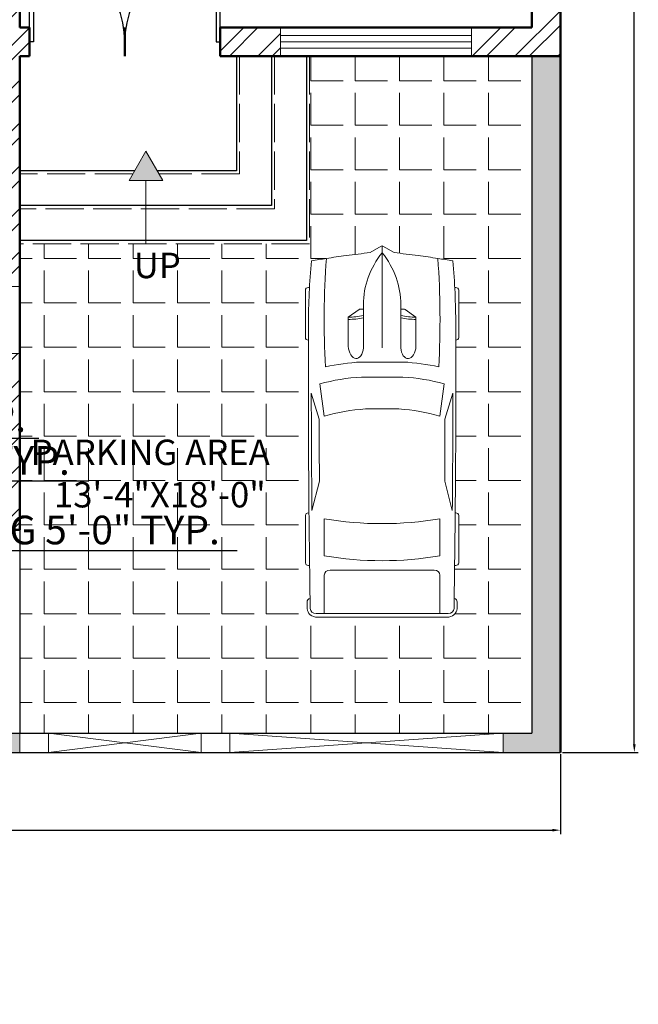
# Model space of a CAD drawing. Units: inches. Extents: x 764 to 1199, y 2696 to 3678.
# Tile 1 of 3: x 984 to 1179, y 2741 to 3051. Entities that reach past the tile are written whole.
import ezdxf

# ---------------------------------------------------------------- set-up
doc = ezdxf.new("R2010")
doc.units = ezdxf.units.IN
doc.linetypes.add('ACAD_ISO02W100', pattern=[15, 12, -3])
for name, color, linetype, lineweight in [('A-ANNO-DIMS', 2, 'Continuous', 18), ('A-ANNO-SYMB', 7, 'Continuous', 18), ('A-ANNO-TEXT', 7, 'Continuous', 18), ('A-AREA-IDEN', 7, 'Continuous', 18), ('A-DOOR', 4, 'Continuous', 25), ('A-FLOR-PATT', 9, 'Continuous', 13), ('A-FLOR-STRS', 7, 'Continuous', 25), ('A-GLAZ', 244, 'Continuous', 20), ('A-STRS-HIDN', 8, 'ACAD_ISO02W100', 13), ('A-WALL', 7, 'Continuous', 50), ('A-WALL-PATT', 252, 'Continuous', 13), ('C-PKG-VEHI', 8, 'Continuous', 18), ('L-GATE', 244, 'Continuous', 20), ('L-HRDS', 7, 'Continuous', 30)]:
    doc.layers.add(name, color=color, linetype=linetype, lineweight=lineweight)
doc.styles.get("Standard").update_dxf_attribs({"font": 'arial.ttf'})
doc.dimstyles.new('ISO-25', dxfattribs={"dimtxt": 9, "dimasz": 2.5, "dimexe": 1.25, "dimexo": 0.625, "dimtad": 1, "dimlunit": 3, "dimtxsty": 'Standard', "dimcen": 2.5, "dimadec": 0, "dimazin": 0, "dimtfac": 1, "dimtmove": 0, "dimatfit": 3, "dimfxl": 1, "dimarcsym": 0})
pattern_1 = [(45, (0, 0), (-6.735192090801866, 6.735192090801866), []), (45, (4.49013, 0), (-6.735192090801866, 6.735192090801866), [])]

# ---------------------------------------------------------------- blocks, each defined once
blk = doc.blocks.new('*U2')
for p, q in [((0, 0), (-1e-16, -5.999999999999999)), ((40, -6e-16), (40, -6))]:
    blk.add_line(p, q)
blk.add_lwpolyline([(0, 0), (5.6e-15, 40), (1.750000000000007, 40), (1.749999999999998, -7e-16)], close=True)
blk.add_arc((0, 0), 40, 0, 90)
blk = doc.blocks.new('*U6')
for p, q in [((0, 0), (0, -5.999999999999999)), ((-40, -6e-16), (-40, -6))]:
    blk.add_line(p, q)
blk.add_lwpolyline([(0, 0), (-7.1e-15, 40), (-1.750000000000007, 40), (-1.75, -7e-16)], close=True)
blk.add_arc((0, 0), 40, 90, 180)
blk = doc.blocks.new('*U11')
for p, q in [((21.10406751471477, 37.40863046792069), (21.10406751471477, 36.83230215753705)), ((46.55368679439944, 38.88847654282876), (22.35054758993934, 38.88847654282876)), ((47.80016686962392, 37.39011648242055), (47.80016686962392, 37.40863046792069)), ((87.98532186932616, 31.87120872459877), (74.75900729854769, 35.92175679182955)), ((134.313356548143, 35.6043097713567), (119.2882629232503, 31.77757799177584)), ((135.4513231603356, 37.07354110333037), (135.4513231603356, 37.40863046792069)), ((136.6978032355602, 38.88847654282876), (160.90094244002, 38.88847654282867)), ((162.1474225152445, 37.40863046792049), (162.1474225152445, 36.77402019194128)), ((70.0302824853563, 31.53613089391356), (86.40615155322342, 29.35124891408057)), ((186.4728846989705, -33.49860931502491), (186.4728846989718, 33.49860931502465)), ((188.3990091454065, -32.75868627757393), (188.3990091454077, 32.75868627757058)), ((138.4228833961707, 29.35124891408074), (157.2465674415997, 29.35124891408074)), ((164.515393597658, 26.39155676426461), (164.5153935976578, -26.39155676426503)), ((186.4728846989718, 29.35124891408083), (167.0083537481071, 29.35124891408083)), ((32.26591480791686, 11.62530558863241), (36.12873726252356, 17.16961494239206)), ((36.12873726252356, 17.16961494239206), (50.93891189819171, 17.16961494239206)), ((32.12291633764599, 9.505833383620029), (32.12291633764599, 11.15369945057711)), ((58.9167604809788, -10.77488335095668), (58.9167604809788, 10.77488335095617)), ((66.55009204259746, -10.5288681329018), (66.55009204259746, 10.52886813290129)), ((186.4728846989718, -10.5288681329018), (186.4728846989718, 10.52886813290129)), ((3.266462181856987, 6.128290093440767), (0.1022408397004821, 0.4060708604429806)), ((29.77279020470884, 9.505833383620029), (51.68362801571248, 9.505833383620029)), ((82.73706193978568, 8.496039918672748), (82.73706193978568, -8.49603991867258)), ((-4.43e-14, -2.558e-13), (51.68362801571248, -2.558e-13)), ((0.1022408397004821, -0.4060708604432933), (3.266462181856987, -6.128290093441194)), ((29.77279020470884, -9.50583338362054), (51.68362801571248, -9.50583338362054)), ((32.12291633764599, -9.50583338362054), (32.12291633764599, -11.15369945057762)), ((32.26591480791686, -11.62530558863292), (36.12873726252356, -17.16961494239257)), ((36.12873726252356, -17.16961494239257), (50.93891189819171, -17.16961494239257)), ((86.40615155322318, -29.35124891408145), (70.03028248535594, -31.53613089391442)), ((157.2465674415997, -29.35124891408117), (138.4228833961707, -29.35124891408126)), ((167.008353748107, -29.35124891408126), (186.4728846989707, -29.35124891408108)), ((87.98532186932607, -31.87120872459903), (74.7590072985476, -35.92175679182964)), ((134.3133565481428, -35.60430977135721), (119.2882629232503, -31.77757799177618)), ((21.10406751471477, -37.4086304679212), (21.10406751471477, -36.83230215753756)), ((46.55368679439944, -38.88847654282927), (22.35054758993934, -38.88847654282927)), ((47.80016686962392, -37.39011648242107), (47.80016686962392, -37.4086304679212)), ((135.4513231603355, -37.07354110333088), (135.4513231603355, -37.4086304679212)), ((136.6978032355602, -38.88847654282927), (160.9009424400199, -38.88847654282918)), ((162.1474225152445, -37.408630467921), (162.1474225152445, -36.77402019194179))]:
    blk.add_line(p, q)
for centre, major_axis, ratio, start_param, end_param in [((266.0300214172791, -27.52442688366631), (1.966072e-10, 313.3077612809058), 0.8423038695435284, 1.367075990158062, 1.391760499156098), ((41.19115208863305, -490.8631038926156), (1.294e-13, 528.2339998381949), 0.8423038695439741, 0.0028100083536837, 0.0755983031096952), ((22.35054758993934, 37.40863046792072), (2.08e-14, -1.479846074908118), 0.842303869543976, 3.141592653589776, 4.712388980384677), ((64.48199294511879, -10555.61767587835), (1.907644e-10, 10593.02630634627), 0.842303869543847, -0.0133969486112073, 0.0027970409639888), ((46.55368679439944, 37.40863046792072), (2.2e-14, 1.479846074908118), 0.8423038695439758, -1.570796326794884, 1.73e-14), ((64.4819929449925, -10555.61767590795), (1.9177683e-09, -10591.54646030096), 0.8423038695482963, 3.133765086725325, 3.140440689641252), ((136.6978032355602, 37.40863046792072), (2.357e-13, -1.479846074908118), 0.842303869543976, 3.141592653589603, 4.712388980384554), ((160.90094244002, 37.40863046792052), (5.59e-14, 1.479846074908118), 0.842303869543976, -1.570796326794865, 4.44e-14), ((180.6280394947615, 35.8381667808375), (7.4e-14, 2.219769112362114), 0.8423038695439693, -0.0130174256259048, 1.249894140392862), ((64.48199294754608, -10556.35759891604), (1.349839377e-06, 10595.3130398087), 0.8423038681351469, -0.0133969484821159, -0.0130174254969711), ((183.9799245485226, 33.49860931502124), (3e-16, -2.959692149816168), 0.8423038695439952, 1.570796326796048, 3.128195704978389), ((183.9799245485216, 32.75868627756583), (8.56e-14, -5.246425615115243), 0.8423038695439737, 1.570796326795794, 3.128195704978164), ((135.2911776514449, 5.387441675478555), (2.2715e-12, 81.77258453065997), 0.8423038695439563, 1.245306111696802, 1.507880129813836), ((95.78879860270445, -3666.353346297651), (1.949864e-10, -3698.236159209632), 0.8423038695446962, 3.134048706297306, 3.14409775411291), ((259.1750197310735, -27.52442688366614), (1.506617e-10, -305.3028914627677), 0.8423038695443789, 4.528606069860317, 4.561837674556238), ((37.47375371777758, -593.9621830607928), (6.21e-14, -623.32820996736), 0.8423038695439826, 3.09604606856106, 3.200911180495224), ((134.4003789125686, 5.387441675477674), (4.276e-13, -89.7774543484738), 0.84230386954398, 4.44948196380473, 4.652344057257214), ((149.595361812917, 2.799442537139299), (8.561e-13, -79.57966406425402), 0.842303869543983, 4.372215489277867, 4.640744122441986), ((17.08207736189386, -1.421e-13), (6.87e-14, 147.0179238898305), 0.8423038695439764, 4.511394369635731, 4.913383591133647), ((35.90576140732288, -1.421e-13), (6.87e-14, 147.0179238898305), 0.8423038695439764, 4.511394369635731, 4.913383591133647), ((167.0083537481071, 26.39155676426464), (1.394e-13, 2.959692149816236), 0.842303869543976, 5.55e-14, 1.57079632679492), ((-204.4946649195746, 52.39684969293512), (4.12053e-11, -250.9602162198571), 0.8423038695441164, 1.385369446298923, 1.434372047871027), ((13.03653510440275, 17.00972444508943), (1.2303e-12, 27.41599049210566), 0.8423038695439277, 4.435146050259648, 4.718221029521873), ((14.20086229321332, 17.00972444508943), (1.2303e-12, 27.41599049210566), 0.8423038695439277, 4.435146050259648, 4.718221029521873), ((50.7902773840875, 13.33772416300607), (6.340077547122382, -0.356608581037027), 0.6038335755719145, -1.39555193967809, 1.581314658479915), ((32.74615637525823, 11.15369945057713), (1.313e-13, 0.7399230374541176), 0.8423038695439091, 0.8797135699495516, 1.570796326795045), ((29.77279020470884, -46.66302566589627), (5.12e-14, 56.16885904951626), 0.842303869543976, 7e-16, 0.5903187773915901), ((0.6232400376122422, -1.421e-13), (1e-16, -0.7399230374541245), 0.842303869543842, 4.131459131953847, 5.293318828815531), ((29.77279020470884, 46.66302566589578), (4.004e-13, 56.16885904951626), 0.8423038695439734, 2.55127387619821, 3.141592653589801), ((-204.4946649195746, -52.39684969293552), (4.02945e-11, 250.9602162198562), 0.8423038695441192, -1.43437204787103, -1.385369446298926), ((13.03653510440275, -17.00972444508983), (1.2568e-12, -27.41599049210552), 0.8423038695439318, 1.564964277657711, 1.848039256919935), ((14.20086229321332, -17.00972444508983), (1.2568e-12, -27.41599049210552), 0.8423038695439318, 1.564964277657711, 1.848039256919935), ((149.5953618129329, -2.799442537137565), (4.0897e-12, -79.57966406427697), 0.8423038695439419, -1.499151468852248, -1.230622835688196), ((32.74615637525823, -11.1536994505777), (1.3e-13, -0.7399230374541176), 0.8423038695439093, 4.712388980384541, 5.403471737230034), ((134.4003789125684, -5.387441675478584), (4.2949e-12, -89.77745434847827), 0.8423038695439354, -1.510751403667474, -1.307889310215002), ((135.2911776514465, -5.387441675480715), (3.2038e-12, -81.77258453066244), 0.8423038695439492, -1.50788012981387, -1.245306111696839), ((259.1750197310694, 27.52442688365929), (1.08535e-11, 305.3028914629043), 0.8423038695439974, 1.721347632622872, 1.754579237318777), ((266.0300214172791, 27.52442688366566), (8.75241e-11, 313.3077612806533), 0.8423038695441819, 1.749832154434603, 1.774516663432659), ((37.47375371777847, 593.9621830607904), (1.1693e-12, -623.3282099673584), 0.8423038695439528, -0.0593185269054384, 0.0455465850287298), ((167.008353748107, -26.39155676426503), (1.02e-14, -2.959692149816192), 0.8423038695439885, 4.712388980384686, 6.283185307179581), ((95.78879860271888, 3666.35334629765), (1.637818e-10, -3698.236159209629), 0.8423038695447546, -0.0025051005232382, 0.007543947292366), ((183.9799245485216, -33.4986093150211), (9.3e-15, 2.959692149816141), 0.8423038695439732, 3.154989602201626, 4.71238898038339), ((183.9799245485177, -32.7586862775633), (2.428e-13, -5.246425615118353), 0.8423038695439808, 0.0133969486110846, 1.570796326792831), ((41.19115208863322, 490.8631038926152), (1.37757e-11, -528.2339998381949), 0.8423038695440652, -0.0755983031097181, -0.0028100083537155), ((22.35054758993934, -37.40863046792117), (2.2e-14, 1.479846074908118), 0.8423038695439758, 1.570796326794908, 3.14159265358981), ((64.48199294495228, 10555.61767590795), (6.117947e-10, 10593.02630637587), 0.8423038695458146, 3.138795612625926, 3.154989602201039), ((46.55368679439944, -37.40863046792117), (2.08e-14, -1.479846074908118), 0.842303869543976, -1.69e-14, 1.570796326794884), ((64.48199294503607, 10555.61767590793), (1.6049794e-09, -10591.54646030094), 0.8423038695397146, 0.0011519639481523, 0.0078275668641468), ((136.6978032355602, -37.40863046792109), (1.56e-14, -1.479846074908162), 0.8423038695440105, -1.570796326794875, -1.27e-14), ((160.9009424400199, -37.408630467921), (1.969e-13, 1.479846074908162), 0.8423038695440109, 3.141592653589951, 4.712388980384771), ((180.6280394947581, -35.83816678083949), (2.274e-13, -2.219769112363032), 0.8423038695439803, -1.249894138785958, 0.0130174256254374), ((64.48199294197605, 10556.3575989598), (9.365289701e-07, 10595.31303985772), 0.8423038705260315, 3.154610079306566, 3.154989602290631)]:
    blk.add_ellipse(centre, major_axis=major_axis, ratio=ratio, start_param=start_param, end_param=end_param)
at = {"extrusion": (0, 0, -1)}
blk.add_ellipse((50.7902773840875, -13.33772416300655), major_axis=(6.340077547122382, 0.3566085810370246), ratio=0.6038335755719145, start_param=-1.39555193967809, end_param=1.581314658479915, dxfattribs=at)
blk = doc.blocks.new('*D14')
at = {"layer": 'A-ANNO-DIMS', "color": 0, "lineweight": -2, "transparency": 16777216}
for p, q in [((777.2372615392014, 2819.625478579777), (777.2372615392014, 2794.515568669596)), ((1154.237261539201, 2819.625478579777), (1154.237261539201, 2794.515568669596)), ((779.7372615392014, 2795.765568669596), (1151.737261539201, 2795.765568669596))]:
    blk.add_line(p, q, dxfattribs=at)
at = {"layer": 'A-ANNO-DIMS', "color": 0, "transparency": 16777216}
for points in [[(779.7372615392014, 2796.182235336263), (779.7372615392014, 2795.34890200293), (777.2372615392014, 2795.765568669596)], [(1151.737261539201, 2796.182235336263), (1151.737261539201, 2795.34890200293), (1154.237261539201, 2795.765568669596)]]:
    blk.add_solid(points, dxfattribs=at)
at = {"layer": 'Defpoints', "color": 0, "transparency": 16777216}
for p in [(777.2372615392014, 2820.250478579778), (1154.237261539201, 2820.250478579778), (1154.237261539201, 2795.765568669596)]:
    blk.add_point(p, dxfattribs=at)
at = {"layer": 'A-ANNO-DIMS', "color": 0, "transparency": 16777216, "insert": (965.7372615392015, 2800.988795136172), "char_height": 9, "attachment_point": 5}
blk.add_mtext('31\'-5"', dxfattribs=at)
blk = doc.blocks.new('*D15')
at = {"layer": 'A-ANNO-DIMS', "color": 0, "lineweight": -2, "transparency": 16777216}
for p, q in [((1154.862261539202, 3551.25047857978), (1178.719991505351, 3551.25047857978)), ((1177.469991505351, 2822.750478579779), (1177.469991505351, 3548.750478579779)), ((1154.862261539202, 2820.250478579778), (1178.719991505351, 2820.250478579778))]:
    blk.add_line(p, q, dxfattribs=at)
at = {"layer": 'A-ANNO-DIMS', "color": 0, "transparency": 16777216}
for points in [[(1177.053324838685, 3548.750478579779), (1177.886658172018, 3548.750478579779), (1177.469991505351, 3551.25047857978)], [(1177.053324838685, 2822.750478579779), (1177.886658172018, 2822.750478579779), (1177.469991505351, 2820.250478579778)]]:
    blk.add_solid(points, dxfattribs=at)
at = {"layer": 'Defpoints', "color": 0, "transparency": 16777216}
for p in [(1154.237261539202, 3551.25047857978), (1177.469991505351, 3551.25047857978), (1154.237261539202, 2820.250478579778)]:
    blk.add_point(p, dxfattribs=at)
at = {"layer": 'A-ANNO-DIMS', "color": 0, "transparency": 16777216, "insert": (1172.249834615857, 3185.750478579778), "char_height": 9, "attachment_point": 5, "rotation": 90}
blk.add_mtext('60\'-11"', dxfattribs=at)
blk = doc.blocks.new('WIN-GLAZING-60IN')
for p, q in [((0.0002615392013468, 4.000478579777791), (60.00026153920135, 4.000478579777791)), ((0.0002615392013468, 2.000478579777791), (60.00026153920135, 2.000478579777791)), ((0.0002615392013468, 0.0004785797777913), (60.00026153920135, 0.0004785797777913))]:
    blk.add_line(p, q)
blk = doc.blocks.new('*D24')
at = {"layer": 'A-ANNO-DIMS', "color": 0, "lineweight": -2, "transparency": 16777216}
for p, q in [((816.2372615392019, 2892.125478579778), (816.2372615392019, 2882.500478579778)), ((876.237261539202, 2892.125478579778), (876.237261539202, 2882.500478579778)), ((818.7372615392019, 2883.750478579778), (873.737261539202, 2883.750478579778)), ((876.237261539202, 2883.750478579778), (1052.558885004413, 2883.750478579778))]:
    blk.add_line(p, q, dxfattribs=at)
at = {"layer": 'A-ANNO-DIMS', "color": 0, "transparency": 16777216}
for points in [[(818.7372615392019, 2884.167145246444), (818.7372615392019, 2883.333811913111), (816.2372615392019, 2883.750478579778)], [(873.737261539202, 2884.167145246444), (873.737261539202, 2883.333811913111), (876.237261539202, 2883.750478579778)]]:
    blk.add_solid(points, dxfattribs=at)
at = {"layer": 'Defpoints', "color": 0, "transparency": 16777216}
for p in [(816.2372615392019, 2892.750478579778), (876.237261539202, 2892.750478579778), (876.237261539202, 2883.750478579778)]:
    blk.add_point(p, dxfattribs=at)
at = {"layer": 'A-ANNO-DIMS', "color": 0, "transparency": 16777216, "insert": (965.6480732718076, 2889.032027010883), "char_height": 9, "attachment_point": 5}
blk.add_mtext('WINDOW GLAZING 5\'-0" TYP.', dxfattribs=at)
blk = doc.blocks.new('*D28')
at = {"layer": 'A-ANNO-DIMS', "color": 0, "lineweight": -2, "transparency": 16777216}
for p, q in [((829.3360851341931, 2919.092989980183), (826.8360851341931, 2919.092989980183)), ((831.8360851341932, 2919.092989980183), (833.8706302982391, 2919.092989980183)), ((831.8360851341932, 2918.77317175479), (831.8360851341932, 2917.842989980183)), ((833.8706302982391, 2918.77317175479), (833.8706302982391, 2917.842989980183)), ((836.3706302982391, 2919.092989980183), (990.1983929176115, 2919.092989980183))]:
    blk.add_line(p, q, dxfattribs=at)
at = {"layer": 'A-ANNO-DIMS', "color": 0, "transparency": 16777216}
for points in [[(829.3360851341931, 2919.50965664685), (829.3360851341931, 2918.676323313516), (831.8360851341932, 2919.092989980183)], [(836.3706302982391, 2919.50965664685), (836.3706302982391, 2918.676323313516), (833.8706302982391, 2919.092989980183)]]:
    blk.add_solid(points, dxfattribs=at)
at = {"layer": 'Defpoints', "color": 0, "transparency": 16777216}
for p in [(831.8360851341932, 2919.39817175479), (833.8706302982391, 2919.39817175479), (833.8706302982391, 2919.092989980183)]:
    blk.add_point(p, dxfattribs=at)
at = {"layer": 'A-ANNO-DIMS', "color": 0, "transparency": 16777216, "insert": (914.5345116079253, 2924.374538411288), "char_height": 9, "attachment_point": 5}
blk.add_mtext('HOB CONTROL 0\'-2" TYP.', dxfattribs=at)
blk = doc.blocks.new('*D32')
at = {"layer": 'A-ANNO-DIMS', "color": 0, "lineweight": -2, "transparency": 16777216}
for p, q in [((828.174202117123, 2906.483577856705), (828.174202117123, 2904.383671295855)), ((838.006912522789, 2906.483577856705), (838.006912522789, 2904.383671295855)), ((830.674202117123, 2905.633671295855), (835.506912522789, 2905.633671295855)), ((838.006912522789, 2905.633671295855), (1005.911755633294, 2905.633671295855))]:
    blk.add_line(p, q, dxfattribs=at)
at = {"layer": 'A-ANNO-DIMS', "color": 0, "transparency": 16777216}
for points in [[(830.674202117123, 2906.050337962522), (830.674202117123, 2905.217004629188), (828.174202117123, 2905.633671295855)], [(835.506912522789, 2906.050337962522), (835.506912522789, 2905.217004629188), (838.006912522789, 2905.633671295855)]]:
    blk.add_solid(points, dxfattribs=at)
at = {"layer": 'Defpoints', "color": 0, "transparency": 16777216}
for p in [(828.174202117123, 2907.108577856705), (838.006912522789, 2907.108577856705), (838.006912522789, 2905.633671295855)]:
    blk.add_point(p, dxfattribs=at)
at = {"layer": 'A-ANNO-DIMS', "color": 0, "transparency": 16777216, "insert": (923.2093340780414, 2910.91215014988), "char_height": 9, "attachment_point": 5}
blk.add_mtext('LARGE BURNER 0\'-10" TYP.', dxfattribs=at)

msp = doc.modelspace()

# ---------------------------------------------------------------- hatches: boundary and pattern name
at = {"layer": 'A-ANNO-SYMB'}
h = msp.add_hatch(color=256, dxfattribs=at)
h.dxf.hatch_style = 1
h.paths.add_polyline_path([(899.8408897103933, 2758.076893952801), (890.7054604401357, 2740.978067102982), (909.2115573473543, 2740.978067102982)])
h.paths.add_polyline_path([(1023.879118762197, 3009.352008593085), (1018.595038768721, 3000.199713573126), (1029.163198755673, 3000.199713573126)])
h.paths.add_polyline_path([(856.904311954004, 3232.137894596994), (851.9031607095966, 3229.250478579777), (856.9043119540038, 3226.363062562561)])
at = {"layer": 'A-FLOR-PATT'}
h = msp.add_hatch(dxfattribs=at)
h.set_pattern_fill('ANGLE', color=256, scale=2)
h.set_pattern_definition([(0, (0, 0), (0, 13.97), [10.16, -3.81]), (90, (0, 0), (-13.97, 9e-16), [10.16, -3.81])])
h.paths.add_polyline_path([(1145.237261539201, 3039.250478579778), (1075.332306219868, 3039.250478579778), (1075.332306219868, 2980.250478579779), (984.2372615392013, 2980.250478579779), (984.2372615392013, 2890.250478579778), (984.2372615392013, 2826.250478579778), (1145.237261539201, 2826.250478579779)])
edge = h.paths.add_edge_path(flags=16)
edge.add_line((1074.044359378595, 2950.710949610617), (1074.044359378595, 2965.718303844056))
edge.add_ellipse((1074.961950029523, 2965.718303844056), major_axis=(-0.9175906509276504, 3.51e-14), ratio=0.8423038695442256, start_angle=-89.99999999999773, end_angle=2.2168933355715126e-12, ccw=False)
edge.add_line((1074.961950029523, 2966.49119399999), (1075.319307107695, 2966.49119399999))
edge.add_ellipse((1402.521155556098, 2954.036033073497), major_axis=(-327.5358079276594, 1.34747e-11), ratio=0.8423038695438808, start_angle=-3.6504275856967183, end_angle=-2.179950313643019, ccw=False)
edge.add_ellipse((1115.224222824117, 2814.622854933398), major_axis=(-194.2690374936818, 2.2839113e-09), ratio=0.8423038695525722, start_angle=-77.87403444704239, end_angle=-76.21947100982851, ccw=False)
edge.add_ellipse((1115.224222824114, 2818.873354742811), major_axis=(-189.3055525545235, 9.27624e-10), ratio=0.8423038695480677, start_angle=-79.79046100257602, end_angle=-77.5553727062752, ccw=False)
edge.add_ellipse((1065.668382226683, 3106.375531467769), major_axis=(155.6099327240636, 1.701453e-10), ratio=0.8423038695429816, start_angle=-80.74343399286117, end_angle=-77.44506735592547)
edge.add_line((1094.357580677959, 2977.551546942022), (1098.04532158585, 2979.590760752253))
edge.add_ellipse((1098.15747702614, 2979.19049843097), major_axis=(-0.4587953254638792, 0), ratio=0.8423038695441263, start_angle=232.0668695401682, end_angle=270.0000000000337, ccw=False)
edge.add_line((1098.333932547395, 2979.555204671612), (1101.957373374321, 2977.551546942022))
edge.add_ellipse((1130.646571825598, 3106.375531467769), major_axis=(-155.6099327240673, 1.73255e-10), ratio=0.8423038695429623, start_angle=77.44506735592653, end_angle=80.7434339928622)
edge.add_ellipse((1081.090731228163, 2818.873354742809), major_axis=(189.3055525545302, 9.338451e-10), ratio=0.8423038695480526, start_angle=77.55537270627212, end_angle=79.7904610025729, ccw=False)
edge.add_ellipse((1081.090731228163, 2814.622854933398), major_axis=(-194.2690374971778, 1.6398418e-09), ratio=0.8423038695379808, start_angle=256.21947101098567, end_angle=257.8740344481995, ccw=False)
edge.add_ellipse((793.793798496182, 2954.036033073497), major_axis=(327.5358079276593, 1.39837e-11), ratio=0.84230386954386, start_angle=2.1799503136427916, end_angle=3.6504275856966046, ccw=False)
edge.add_line((1120.995646944585, 2966.49119399999), (1121.353004022757, 2966.49119399999))
edge.add_ellipse((1121.353004022757, 2965.718303844056), major_axis=(-0.9175906509274225, 2.376e-13), ratio=0.8423038695444347, start_angle=180.0000000000149, end_angle=270.0000000000149, ccw=False)
edge.add_line((1122.270594673684, 2965.718303844056), (1122.270594673684, 2950.710949610617))
edge.add_ellipse((1121.353004022757, 2950.710949610617), major_axis=(0.9175906509274225, 2.38e-13), ratio=0.8423038695444345, start_angle=269.9999999999851, end_angle=359.9999999999851, ccw=False)
edge.add_ellipse((-5446.939515411542, 2939.594356885331), major_axis=(6568.292519434296, 1.433307e-10), ratio=0.8423038695440498, start_angle=-0.38386677879378794, end_angle=0.09022908859310519, ccw=False)
edge.add_line((1121.145229124143, 2895.589243777794), (1121.353004022757, 2895.589243777794))
edge.add_ellipse((1121.353004022757, 2894.81635362186), major_axis=(-0.9175906509274225, 2.376e-13), ratio=0.8423038695444347, start_angle=180.0000000000149, end_angle=270.0000000000149, ccw=False)
edge.add_line((1122.270594673684, 2894.81635362186), (1122.270594673684, 2879.808999388421))
edge.add_ellipse((1121.353004022757, 2879.808999388421), major_axis=(0.9175906509276499, 6.123e-13), ratio=0.8423038695437304, start_angle=269.99999999996174, end_angle=359.99999999996174, ccw=False)
edge.add_line((1121.353004022757, 2879.036109232487), (1120.959508735578, 2879.036109232487))
edge.add_ellipse((-5446.939515411542, 2939.594356885331), major_axis=(6568.292519434296, 1.433307e-10), ratio=0.8423038695440498, start_angle=-0.61864319632042, end_angle=-0.5282714718192096, ccw=False)
edge.add_ellipse((1120.379225180942, 2867.577051664739), major_axis=(1.37638597639141, 1.5924e-12), ratio=0.842303869543708, start_angle=-0.628237216249488, end_angle=68.46475660093631, ccw=False)
edge.add_ellipse((-5447.398310737152, 2939.594356883826), major_axis=(-6569.710427198919, 2.6897132456e-06), ratio=0.8423038650326489, start_angle=179.3534459264088, end_angle=179.3717628072419, ccw=False)
edge.add_ellipse((1118.469768131707, 2865.49868794809), major_axis=(-3.253089072466935, 4.372e-13), ratio=0.8423038695440137, start_angle=90.00000000006952, end_angle=179.3534459029254, ccw=False)
edge.add_line((1118.46976813171, 2862.75859843438), (1077.845185920569, 2862.758598434381))
edge.add_ellipse((1077.845185920575, 2865.498687948093), major_axis=(3.253089072468953, 1.5619e-12), ratio=0.8423038695439101, start_angle=180.6465540970303, end_angle=269.9999999998346, ccw=False)
edge.add_ellipse((7643.713264816572, 2939.594356887278), major_axis=(6569.710427228598, 1.5974499279e-06), ratio=0.8423038668581472, start_angle=180.6282372023114, end_angle=180.6465540831445, ccw=False)
edge.add_ellipse((1075.935728871337, 2867.577051664742), major_axis=(1.376385976391853, 1.0126e-12), ratio=0.8423038695440634, start_angle=111.53524350398621, end_angle=180.6282372161408, ccw=False)
edge.add_ellipse((7643.254469482177, 2939.594356885431), major_axis=(-6568.292519452651, 2.27921e-10), ratio=0.8423038695440235, start_angle=0.5282714718193802, end_angle=0.6465540970629036, ccw=False)
edge.add_line((1075.355445316702, 2879.036109232487), (1074.961950029523, 2879.036109232487))
edge.add_ellipse((1074.961950029523, 2879.808999388421), major_axis=(-0.9175906509274225, 2.376e-13), ratio=0.8423038695444347, start_angle=1.4779288903810084e-11, end_angle=90.00000000001478, ccw=False)
edge.add_line((1074.044359378596, 2879.808999388421), (1074.044359378595, 2894.81635362186))
edge.add_ellipse((1074.961950029523, 2894.81635362186), major_axis=(-0.9175906509276504, 3.51e-14), ratio=0.8423038695442256, start_angle=-89.99999999999773, end_angle=2.2168933355715126e-12, ccw=False)
edge.add_line((1074.961950029523, 2895.589243777794), (1075.169724928137, 2895.589243777794))
edge.add_ellipse((7643.254469482177, 2939.594356885431), major_axis=(-6568.292519452651, 2.27921e-10), ratio=0.8423038695440235, start_angle=-0.09022908859117251, end_angle=0.3838667787944132, ccw=False)
edge.add_ellipse((1074.961950029523, 2950.710949610617), major_axis=(0.9175906509276504, 3.57e-14), ratio=0.8423038695442258, start_angle=179.9999999999978, end_angle=269.9999999999977, ccw=False)
edge = h.paths.add_edge_path(flags=0)
edge.add_line((1075.883898201988, 2933.222010159516), (1078.395473629086, 2925.020925734477))
edge.add_ellipse((3371.509828059429, 2920.182316221841), major_axis=(-2293.12154970155, 1.452554e-10), ratio=0.8423038695547603, start_angle=-0.120897369029341, end_angle=0.3640763488936895)
edge.add_line((1078.453530130051, 2905.611281350079), (1076.08073382097, 2896.294849274287))
edge.add_ellipse((7643.254469482167, 2939.594356885379), major_axis=(6567.374928801716, 7.57234e-10), ratio=0.8423038695393193, start_angle=180.0555943134924, end_angle=180.377764193903, ccw=False)
edge = h.paths.add_edge_path(flags=0)
edge.add_ellipse((1094.816949793167, 2895.688543309169), major_axis=(50.70375922185087, 1.93565e-11), ratio=0.84230386954371, start_angle=94.277420963032, end_angle=111.8349537966862, ccw=False)
edge.add_line((1091.628966306402, 2938.312015140999), (1104.685987745878, 2938.312015140999))
edge.add_ellipse((1101.498004259112, 2895.688543309169), major_axis=(-50.70375922183369, 3.2793e-12), ratio=0.8423038695439737, start_angle=248.1650462032939, end_angle=265.7225790369482, ccw=False)
edge.add_line((1117.711712676277, 2936.154094619487), (1116.356958751482, 2926.000103192763))
edge.add_ellipse((1099.893294246217, 2886.819117036894), major_axis=(49.34402096775494, 2.9723e-12), ratio=0.842303869543992, start_angle=67.20808512240657, end_angle=85.1299304028607)
edge.add_line((1103.425516000914, 2928.275152188595), (1092.889438051367, 2928.275152188595))
edge.add_ellipse((1096.421659806065, 2886.819117036885), major_axis=(-49.3440209677642, 3.1585e-12), ratio=0.8423038695440276, start_angle=-85.12993040286065, end_angle=-67.20808512240966)
edge.add_line((1079.957995300798, 2926.000103192763), (1078.603241376003, 2936.154094619488))
edge = h.paths.add_edge_path(flags=0)
edge.add_line((1087.511316984026, 2957.175024752644), (1091.076375585367, 2959.658866749648))
edge.add_line((1091.076375585367, 2959.658866749648), (1092.263307362159, 2959.658866749648))
edge.add_line((1092.263307362159, 2959.658866749648), (1092.263307362159, 2961.116081661823))
edge.add_ellipse((1127.091267385166, 2961.116081661825), major_axis=(-34.82796002300756, 6.672e-13), ratio=0.8423038695439766, start_angle=-29.43856959797853, end_angle=1.1937117960769683e-12, ccw=False)
edge.add_ellipse((1069.223686667114, 2961.116081661825), major_axis=(34.82796002300779, 6.44e-13), ratio=0.8423038695439737, start_angle=-1.0800249583553523e-12, end_angle=29.43856959797853, ccw=False)
edge.add_line((1104.051646690121, 2961.116081661825), (1104.051646690121, 2959.658866749648))
edge.add_line((1104.051646690121, 2959.658866749648), (1105.238578466913, 2959.658866749648))
edge.add_line((1105.238578466913, 2959.658866749648), (1108.803637068254, 2957.175024752644))
edge.add_line((1108.803637068254, 2957.175024752644), (1108.803637068254, 2947.991854952273))
edge.add_ellipse((1106.427641879188, 2948.084016997272), major_axis=(0.2211180646092897, 3.931216889403082), ratio=0.60383357557183, start_angle=106.34259195433219, end_angle=270.9979857250065, ccw=False)
edge.add_line((1104.051646690121, 2947.530087638348), (1104.051646690121, 2961.116081661825))
edge.add_ellipse((1069.223686667114, 2961.116081661825), major_axis=(34.82796002300779, 6.44e-13), ratio=0.8423038695439737, start_angle=-1.0609e-12, end_angle=29.43856959797842)
edge.add_ellipse((1127.091267385166, 2961.116081661825), major_axis=(-34.82796002300756, 6.672e-13), ratio=0.8423038695439766, start_angle=-29.43856959797857, end_angle=1.093e-12)
edge.add_line((1092.263307362159, 2961.116081661823), (1092.263307362159, 2947.530087638348))
edge.add_ellipse((1089.887312173092, 2948.084016997272), major_axis=(-0.2211180646050052, 3.931216889402904), ratio=0.6038335755719598, start_angle=89.00201427505539, end_angle=253.6574080457286, ccw=False)
edge.add_line((1087.511316984026, 2947.991854952273), (1087.511316984026, 2957.175024752644))
edge = h.paths.add_edge_path(flags=0)
edge.add_ellipse((1098.15747702614, 2968.985061858902), major_axis=(91.15966502695917, 2.687e-13), ratio=0.8423038695440146, start_angle=256.4018653097692, end_angle=283.5981346902303)
edge.add_line((1116.356958751482, 2893.746703572226), (1116.356958751482, 2882.074924466975))
edge.add_ellipse((1098.15747702614, 2957.313282753651), major_axis=(91.15966502695917, 2.687e-13), ratio=0.8423038695440146, start_angle=256.4018653097692, end_angle=283.59813469023027, ccw=False)
edge.add_line((1079.957995300799, 2882.074924466975), (1079.957995300798, 2893.746703572226))
edge = h.paths.add_edge_path(flags=0)
edge.add_ellipse((1081.793176602654, 2876.022049101704), major_axis=(1.8351813018553, 5.771e-13), ratio=0.8423038695439778, start_angle=89.99999999998198, end_angle=179.999999999982, ccw=False)
edge.add_line((1081.793176602654, 2877.567829413571), (1114.521777449627, 2877.567829413571))
edge.add_ellipse((1114.521777449627, 2876.022049101704), major_axis=(1.835181301855073, 8.16e-14), ratio=0.8423038695440823, start_angle=-2.5011104298755527e-12, end_angle=89.9999999999975, ccw=False)
edge.add_line((1116.356958751482, 2876.022049101704), (1116.356958751482, 2863.952907636222))
edge.add_line((1116.356958751482, 2863.952907636222), (1118.928563457174, 2863.952907636222))
edge.add_ellipse((1118.928563457171, 2865.49868794809), major_axis=(1.835181301855095, 1.137e-12), ratio=0.8423038695438243, start_angle=-89.99999999995973, end_angle=-0.6465540970936243)
edge.add_line((1118.928563457174, 2863.952907636222), (1077.386390595101, 2863.952907636223))
edge.add_ellipse((1077.386390595109, 2865.49868794809), major_axis=(-1.835181301855106, 5.282e-13), ratio=0.8423038695440666, start_angle=0.6465540971030157, end_angle=89.99999999992379)
edge.add_line((1077.386390595102, 2863.952907636223), (1079.957995300799, 2863.952907636223))
edge.add_line((1079.957995300799, 2863.952907636223), (1079.957995300798, 2876.022049101704))
edge = h.paths.add_edge_path(flags=0)
edge.add_line((1117.919480423195, 2925.020925734481), (1120.431055850292, 2933.222010159514))
edge.add_ellipse((-5446.939515429896, 2939.59435688541), major_axis=(6567.374928801726, 1.2049168e-09), ratio=0.842303869546702, start_angle=-0.37776419392042726, end_angle=-0.05559431350991417, ccw=False)
edge.add_line((1120.23422023131, 2896.294849274289), (1117.861423922229, 2905.611281350081))
edge.add_ellipse((-1175.194874007148, 2920.182316221851), major_axis=(2293.121549701552, 1.488196e-10), ratio=0.8423038695464983, start_angle=-0.3640763488940512, end_angle=0.1208973690289373)
h.paths.add_polyline_path([(1017.188004896857, 2965.065032736347), (1036.713243641741, 2965.065032736347), (1036.713243641741, 2981.550708043304), (1017.188004896857, 2981.550708043304)], flags=24)
h.paths.add_polyline_path([(984.7711821396424, 2892.771077568815), (1072.6292994657, 2892.771077568815), (1072.6292994657, 2922.62282836463), (984.7711821396424, 2922.62282836463)], flags=24)
at = {"layer": 'A-WALL-PATT'}
h = msp.add_hatch(dxfattribs=at)
h.set_pattern_fill('ANSI32', color=256)
h.set_pattern_definition(pattern_1)
h.paths.add_polyline_path([(975.2372615392017, 2999.250478579778), (960.2372615392013, 2999.250478579778), (960.2372615392013, 2993.250478579778), (975.2372615392017, 2993.250478579778), (975.2372615392015, 2966.770834040433), (984.2372615392013, 2966.770834040433), (984.2372615392013, 3039.250478579778), (987.2372615392013, 3039.250478579779), (987.2372615392013, 3043.750478579778), (987.2372615392013, 3048.250478579778), (984.2372615392013, 3048.250478579778), (984.2372615392013, 3053.250478579777), (984.2372615392013, 3077.250478579778), (975.2372615392014, 3077.250478579778), (975.2372615392014, 3053.250478579777), (915.2372615392017, 3053.250478579777), (906.2372615392017, 3053.250478579777), (906.2372615392017, 3047.250478579778), (906.2372615392017, 2990.250478579778), (910.7372615392017, 2990.250478579778), (915.2372615392017, 2990.250478579778), (915.2372615392017, 2993.250478579778), (930.2372615392014, 2993.250478579778), (930.2372615392014, 2999.250478579778), (915.2372615392017, 2999.250478579778), (915.2372615392017, 3047.250478579778), (975.237261539201, 3047.250478579778)])
h.paths.add_polyline_path([(1047.237261539201, 3048.250478579778), (1047.237261539201, 3043.750478579778), (1047.237261539201, 3039.250478579779), (1066.237261539201, 3039.250478579778), (1066.237261539201, 3048.250478579778)])
h.paths.add_polyline_path([(906.2372615392014, 2899.250478579777), (876.2372615392013, 2899.250478579777), (876.2372615392013, 2890.250478579778), (984.2372615392013, 2890.250478579778), (984.2372615392013, 2945.770834040434), (975.2372615392015, 2945.770834040434), (975.2372615392014, 2899.250478579777), (915.2372615392014, 2899.250478579777), (915.2372615392017, 2960.250478579777), (906.2372615392012, 2960.250478579777)])
h.paths.add_polyline_path([(786.2372615392021, 3047.250478579778), (846.2372615392014, 3047.250478579778), (846.2372615392014, 3053.250478579777), (786.2372615392015, 3053.250478579777), (786.2372615392015, 3247.250478579778), (915.2372615392019, 3247.250478579778), (915.2372615392019, 3259.250478579777), (906.2372615392019, 3259.250478579777), (906.2372615392019, 3256.250478579777), (839.2372615392017, 3256.250478579777), (839.2372615392017, 3271.750478579777), (830.2372615392014, 3271.750478579777), (830.2372615392014, 3256.250478579777), (786.2372615392015, 3256.250478579777), (786.2372615392015, 3308.250478579778), (830.2372615392014, 3308.250478579778), (830.2372615392014, 3292.750478579777), (839.2372615392017, 3292.750478579777), (839.2372615392017, 3308.250478579778), (906.2372615392018, 3308.250478579777), (906.2372615392018, 3289.250478579778), (915.2372615392019, 3289.250478579778), (915.2372615392017, 3320.250478579777), (906.2372615392018, 3320.250478579777), (906.2372615392018, 3317.250478579778), (786.2372615392015, 3317.250478579778), (786.2372615392015, 3336.750478579778), (777.2372615392014, 3336.750478579778), (777.2372615392014, 2890.250478579778), (816.2372615392014, 2890.250478579778), (816.2372615392014, 2899.250478579777), (786.2372615392014, 2899.250478579777)])
h.paths.add_polyline_path([(979.2372615392013, 3443.250478579778), (997.7372615392013, 3443.250478579778), (997.7372615392013, 3452.250478579777), (979.2372615392014, 3452.250478579777), (979.2372615392014, 3455.250478579777), (970.2372615392011, 3455.250478579777), (970.2372615392011, 3386.250478579778), (967.2372615392012, 3386.250478579778), (967.2372615392012, 3377.250478579777), (970.2372615392011, 3377.250478579777), (970.2372615392011, 3290.250478579777), (979.2372615392013, 3290.250478579777)])
h.paths.add_polyline_path([(777.2372615392014, 3357.750478579777), (786.2372615392014, 3357.750478579777), (786.2372615392014, 3377.250478579777), (906.2372615392014, 3377.250478579777), (906.2372615392017, 3350.250478579777), (915.2372615392017, 3350.250478579777), (915.2372615392014, 3377.250478579777), (931.2372615392012, 3377.250478579777), (931.2372615392012, 3386.250478579778), (786.2372615392014, 3386.250478579778), (786.2372615392014, 3542.250478579778), (970.2372615392015, 3542.250478579778), (970.2372615392015, 3485.250478579778), (979.2372615392014, 3485.250478579778), (979.2372615392014, 3542.250478579778), (979.2372615392014, 3551.250478579778), (777.2372615392014, 3551.250478579778)])
h.paths.add_polyline_path([(1076.237261539201, 3452.250478579778), (1057.737261539201, 3452.250478579778), (1057.737261539201, 3443.250478579777), (1076.237261539201, 3443.250478579777), (1088.237261539201, 3443.250478579777), (1088.237261539201, 3452.250478579777), (1085.237261539201, 3452.250478579777), (1085.237261539201, 3517.522907527973), (1076.237261539201, 3517.522907527973)])
h.paths.add_polyline_path([(913.697357037155, 2904.723445549297), (949.0861701340172, 2904.723445549297), (949.0861701340172, 2931.714123130015), (913.697357037155, 2931.714123130015)], flags=24)
h = msp.add_hatch(color=256, dxfattribs=at)
h.dxf.hatch_style = 1
h.paths.add_polyline_path([(1076.237261539201, 3551.250478579778), (979.2372615392014, 3551.250478579778), (979.2372615392014, 3542.250478579778), (1076.237261539201, 3542.250478579778)])
h.paths.add_polyline_path([(786.2372615392014, 2826.250478579777), (786.2372615392015, 2890.250478579778), (777.2372615392014, 2890.250478579778), (777.2372615392014, 2820.250478579778), (984.2372615392013, 2820.250478579778), (984.2372615392013, 2826.250478579778)])
h.paths.add_polyline_path([(1154.237261539201, 3039.250478579778), (1145.237261539201, 3039.250478579778), (1145.237261539201, 2826.250478579779), (1136.237261539201, 2826.250478579779), (1136.237261539201, 2820.250478579778), (1154.237261539201, 2820.250478579778)])
h = msp.add_hatch(dxfattribs=at)
h.set_pattern_fill('ANSI32', color=256)
h.set_pattern_definition(pattern_1)
h.paths.add_polyline_path([(1154.237261539201, 3551.250478579778), (1076.237261539201, 3551.250478579778), (1076.237261539201, 3542.250478579778), (1076.237261539201, 3538.522907527973), (1085.237261539201, 3538.522907527973), (1085.237261539201, 3542.250478579778), (1145.237261539201, 3542.250478579778), (1145.237261539201, 3452.250478579777), (1118.237261539201, 3452.250478579777), (1118.237261539201, 3443.250478579777), (1145.237261539201, 3443.250478579777), (1145.237261539201, 3251.250478579777), (979.2372615392014, 3251.250478579778), (979.2372615392013, 3254.250478579777), (970.2372615392011, 3254.250478579777), (970.2372615392011, 3242.250478579778), (1145.237261539201, 3242.250478579777), (1145.237261539201, 3048.250478579777), (1126.237261539201, 3048.250478579777), (1126.237261539201, 3039.250478579778), (1154.237261539201, 3039.250478579778)])

# ---------------------------------------------------------------- linework, layer by layer
at = {"layer": 'A-ANNO-SYMB'}
msp.add_line((1023.879118762197, 2980.250478579779), (1023.879118762197, 3000.199713573126), dxfattribs=at)
msp.add_lwpolyline([(1023.879118762197, 3009.352008593085), (1018.595038768721, 3000.199713573126), (1029.163198755673, 3000.199713573126)], close=True, dxfattribs=at)
at = {"layer": 'A-FLOR-STRS'}
for p, q in [((1052.332306219869, 3039.250478579779), (1052.332306219869, 3003.250478579779)), ((1063.332306219868, 3039.250478579779), (1063.332306219868, 2992.250478579779)), ((1074.332306219869, 3039.250478579779), (1074.332306219869, 2981.250478579779)), ((1020.356398766546, 3003.250478579779), (984.2372615392013, 3003.250478579779)), ((1052.332306219869, 3003.250478579779), (1027.401838757848, 3003.250478579779)), ((1063.332306219868, 2992.250478579779), (984.2372615392013, 2992.250478579779)), ((1074.332306219869, 2981.250478579779), (984.2372615392013, 2981.250478579779))]:
    msp.add_line(p, q, dxfattribs=at)
at = {"layer": 'A-GLAZ'}
for points in [[(1066.237261539201, 3048.250478579778), (1126.237261539201, 3048.250478579778), (1126.237261539201, 3039.250478579778), (1066.237261539201, 3039.250478579778)], [(984.2372615392013, 2966.770834040433), (984.2372615392013, 2945.770834040434), (975.2372615392014, 2945.770834040434), (975.2372615392014, 2966.770834040433)]]:
    msp.add_lwpolyline(points, close=True, dxfattribs=at)
at = {"layer": 'A-STRS-HIDN'}
for p, q in [((1053.332306219869, 3039.250478579779), (1053.332306219869, 3002.250478579779)), ((1064.332306219869, 3039.250478579779), (1064.332306219869, 2991.250478579779)), ((1075.332306219868, 3039.250478579779), (1075.332306219868, 2980.250478579779)), ((1019.779048497357, 3002.250478579779), (984.2372615392013, 3002.250478579779)), ((1053.332306219869, 3002.250478579779), (1027.979189027037, 3002.250478579779)), ((1064.332306219869, 2991.250478579779), (984.2372615392013, 2991.250478579779)), ((1075.332306219868, 2980.250478579779), (984.2372615392013, 2980.250478579779))]:
    msp.add_line(p, q, dxfattribs=at)
at = {"layer": 'A-WALL'}
for p, q in [((1154.237261539201, 3551.250478579778), (1154.237261539201, 2820.250478579778)), ((1145.237261539201, 3242.250478579777), (1145.237261539201, 3048.250478579777)), ((984.2372615392013, 3053.250478579777), (984.2372615392013, 3048.250478579777)), ((984.2372615392013, 3048.250478579778), (987.2372615392017, 3048.250478579778)), ((987.2372615392013, 3039.250478579778), (987.2372615392015, 3048.250478579777)), ((1017.237261539201, 3039.250478579778), (1017.237261539201, 3048.250478579777)), ((1047.237261539201, 3039.250478579777), (1047.237261539201, 3048.250478579777)), ((1047.237261539201, 3048.250478579778), (1145.237261539201, 3048.250478579777)), ((984.2372615392013, 3039.250478579778), (987.2372615392015, 3039.250478579779)), ((984.2372615392013, 3039.250478579778), (984.2372615392013, 2890.250478579778)), ((1047.237261539201, 3039.250478579779), (1154.237261539201, 3039.250478579778)), ((777.2372615392014, 2890.250478579778), (984.2372615392013, 2890.250478579778))]:
    msp.add_line(p, q, dxfattribs=at)
at = {"layer": 'L-GATE'}
for p, q in [((984.2372615392013, 2826.250478579778), (984.2372615392013, 2820.250478579778)), ((993.2372615392013, 2826.250478579778), (993.2372615392013, 2820.250478579778)), ((993.2372615392013, 2820.250478579778), (1041.237261539201, 2826.250478579778)), ((1041.237261539201, 2820.250478579778), (993.2372615392013, 2826.250478579778)), ((1041.237261539201, 2826.250478579778), (1041.237261539201, 2820.250478579776)), ((1050.237261539201, 2826.250478579778), (1050.237261539201, 2820.250478579776)), ((1050.237261539201, 2820.250478579778), (1136.237261539201, 2826.250478579779)), ((1136.237261539201, 2820.250478579778), (1050.237261539201, 2826.250478579778)), ((1136.237261539201, 2826.250478579779), (1136.237261539201, 2820.250478579778))]:
    msp.add_line(p, q, dxfattribs=at)
at = {"layer": 'L-HRDS'}
for p, q in [((1145.237261539201, 3039.250478579778), (1145.237261539201, 2826.25047857978)), ((984.2372615392013, 2890.250478579778), (984.2372615392013, 2826.250478579779)), ((786.2372615392014, 2826.250478579777), (1145.237261539201, 2826.250478579779)), ((777.2372615392014, 2820.250478579778), (1154.237261539201, 2820.250478579778))]:
    msp.add_line(p, q, dxfattribs=at)

# ---------------------------------------------------------------- block references
at = {"layer": 'A-DOOR', "xscale": 0.75, "yscale": 0.75, "zscale": 0.75}
for name, p in [('*U2', (987.2372615392013, 3043.750478579778)), ('*U6', (1047.237261539201, 3043.750478579778))]:
    msp.add_blockref(name, p, dxfattribs=at)
at = {"layer": 'A-GLAZ'}
msp.add_blockref('WIN-GLAZING-60IN', (1066.237, 3041.75), dxfattribs=at)
at = {"layer": 'C-PKG-VEHI', "xscale": 0.6200581712422676, "yscale": 0.6200581712422676, "zscale": 0.6200581712422676, "rotation": 270}
msp.add_blockref('*U11', (1098.15747702614, 2979.576943508937), dxfattribs=at)

# ---------------------------------------------------------------- texts
at = {"layer": 'A-ANNO-TEXT', "insert": (1020.066586070117, 2977.433381986006), "char_height": 8, "attachment_point": 1}
msp.add_mtext_dynamic_manual_height_columns('UP', width=15.69326219501272, gutter_width=12.5, heights=[0], dxfattribs=at)
at = {"layer": 'A-AREA-IDEN', "insert": (987.6333922351404, 2918.641927955354), "char_height": 8, "attachment_point": 1}
msp.add_mtext_dynamic_manual_height_columns('PARKING AREA\\P   13\'-4"X18\'-0"', width=86.6462664767405, gutter_width=12.5, heights=[0], dxfattribs=at)

# ---------------------------------------------------------------- dimensions: what is measured, and where the dimension line sits
at = {"layer": 'A-ANNO-DIMS'}
dim = msp.add_linear_dim(base=(1177.469991505351, 3551.25047857978), p1=(1154.237261539201, 2820.250478579778), p2=(1154.237261539201, 3551.250478579778), angle=90, dimstyle='ISO-25', override={"dimclrd": 0, "dimclre": 0, "dimclrt": 0}, dxfattribs=at)
dim.commit()
dim.dimension.update_dxf_attribs({"geometry": '*D15', "text_midpoint": (1172.249834615857, 3185.750478579778)})
for base, p1, p2, text, picture, middle in [((833.8706302982391, 2919.092989980183), (831.8360851341932, 2919.39817175479), (833.8706302982391, 2919.39817175479), 'HOB CONTROL <> TYP.', '*D28', (914.5345116079253, 2924.374538411288)), ((838.006912522789, 2905.633671295855), (828.174202117123, 2907.108577856705), (838.006912522789, 2907.108577856705), 'LARGE BURNER <> TYP.', '*D32', (923.2093340780414, 2910.91215014988)), ((876.237261539202, 2883.750478579778), (816.2372615392019, 2892.750478579778), (876.237261539202, 2892.750478579778), 'WINDOW GLAZING <> TYP.', '*D24', (965.6480732718076, 2889.032027010883))]:
    dim = msp.add_linear_dim(base=base, p1=p1, p2=p2, text=text, dimstyle='ISO-25', override={"dimdec": 1, "dimlfac": 1, "dimrnd": 0, "dimzin": 1, "dimdsep": 46, "dimlunit": 4, "dimfrac": 2}, dxfattribs=at)
    dim.commit()
    dim.dimension.update_dxf_attribs({"geometry": picture, "text_midpoint": middle})
dim = msp.add_linear_dim(base=(1154.237261539201, 2795.765568669596), p1=(777.2372615392014, 2820.250478579778), p2=(1154.237261539201, 2820.250478579778), dimstyle='ISO-25', override={"dimclrd": 0, "dimclre": 0, "dimclrt": 0}, dxfattribs=at)
dim.commit()
dim.dimension.update_dxf_attribs({"geometry": '*D14', "text_midpoint": (965.7372615392015, 2800.988795136172)})

doc.saveas('drawing.dxf')
